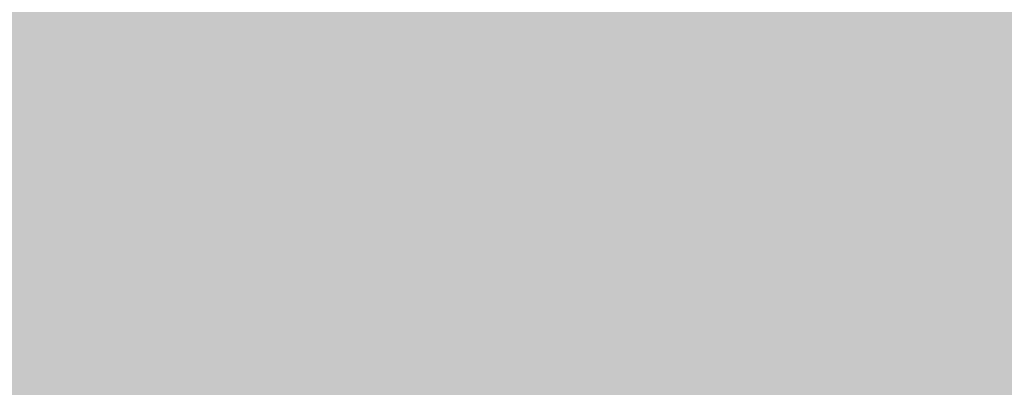
# Model space of a CAD drawing. Units: feet. Extents: x 3168 to 4724, y 827 to 1477.
# Tile 28 of 256: x 3261.901 to 3270.273, y 1093.654 to 1096.781. Entities that reach past the tile are written whole.
import ezdxf

# ---------------------------------------------------------------- set-up
doc = ezdxf.new("R2010")
doc.units = ezdxf.units.FT
doc.layers.add('A-ELEV-PATT', color=8, linetype='Continuous', lineweight=13)

msp = doc.modelspace()

# ---------------------------------------------------------------- hatches: boundary and pattern name
at = {"layer": 'A-ELEV-PATT'}
h = msp.add_hatch(color=256, dxfattribs=at)
h.dxf.hatch_style = 1
edge = h.paths.add_edge_path()
edge.add_ellipse((3552.9058, 979.2201), major_axis=(36.7449, 0), ratio=0.4848485, start_angle=0, end_angle=360)
edge = h.paths.add_edge_path()
edge.add_ellipse((3559.8916, 929.2523), major_axis=(36.7449, 0), ratio=0.4848485, start_angle=0, end_angle=360)
edge = h.paths.add_edge_path()
edge.add_line((3299.3168, 1198.6061), (3479.9167, 1198.6061))
edge.add_line((3479.9167, 1198.6061), (3479.9167, 1209.8686))
edge.add_spline(control_points=[(3479.9167, 1209.8686), (3464.3012, 1209.8686), (3448.6856, 1209.8686), (3410.9491, 1209.8686), (3388.8282, 1209.8686), (3355.6469, 1209.8686), (3344.5864, 1209.8686), (3327.9957, 1209.8686), (3322.4655, 1209.8686), (3314.1702, 1209.8686), (3311.4051, 1209.8686), (3307.2574, 1209.8686), (3305.8748, 1209.8686), (3303.801, 1209.8686), (3303.1097, 1209.8686), (3302.0728, 1209.8686), (3301.7272, 1209.8686), (3301.2087, 1209.8686), (3301.0359, 1209.8686), (3300.7767, 1209.8686), (3300.6903, 1209.8686), (3300.5606, 1209.8686), (3300.5174, 1209.8686), (3300.4526, 1209.8686), (3300.431, 1209.8686), (3300.3986, 1209.8686), (3300.3878, 1209.8686), (3300.3662, 1209.8686), (3300.3457, 1209.8686), (3300.3455, 1209.8686), (3300.3455, 1209.8686), (3300.3433, 1209.8686), (3300.3411, 1209.8686), (3300.3379, 1209.8686), (3300.3368, 1209.8686), (3300.3339, 1209.8686), (3300.3321, 1209.8686), (3300.3255, 1209.8686), (3300.3207, 1209.8686), (3300.3109, 1209.8686), (3300.306, 1209.8686), (3300.2905, 1209.8686), (3300.28, 1209.8686), (3300.2324, 1209.8688), (3300.1953, 1209.869), (3299.9511, 1209.8706), (3299.7448, 1209.8743), (3299.4368, 1209.8833), (3299.3344, 1209.8868), (3299.1811, 1209.8929), (3299.13, 1209.8951), (3298.6522, 1209.9168), (3298.2295, 1209.9457), (3297.6016, 1210.0024), (3297.3934, 1210.0235), (3297.0827, 1210.0583), (3296.9793, 1210.0705), (3296.293, 1210.1549), (3295.7181, 1210.2434), (3294.8687, 1210.3989), (3294.5877, 1210.4545), (3294.1693, 1210.5433), (3294.0304, 1210.5739), (3291.7071, 1211.1012), (3289.6536, 1211.8134), (3285.7763, 1213.564), (3283.9514, 1214.6035), (3280.5122, 1216.9801), (3278.8972, 1218.3176), (3276.3799, 1220.8295), (3275.416, 1221.9177), (3274.0393, 1223.7077), (3273.581, 1224.3495), (3273.1432, 1225.0163)], knot_values=[39.119033, 39.119033, 39.119033, 39.119033, 39.286353, 39.286353, 39.523379, 39.523379, 39.641892, 39.641892, 39.701148, 39.701148, 39.730777, 39.730777, 39.745591, 39.745591, 39.752998, 39.752998, 39.756701, 39.756701, 39.758553, 39.758553, 39.759479, 39.759479, 39.759942, 39.759942, 39.760173, 39.760173, 39.760289, 39.760289, 39.760405, 39.760405, 39.760463, 39.760463, 39.763389, 39.763389, 39.764851, 39.764851, 39.767304, 39.767304, 39.773825, 39.773825, 39.78057, 39.78057, 39.79477, 39.79477, 39.845194, 39.845194, 40.126715, 40.126715, 40.267476, 40.267476, 40.337856, 40.337856, 40.927023, 40.927023, 41.221606, 41.221606, 41.368898, 41.368898, 42.202622, 42.202622, 42.619485, 42.619485, 42.827916, 42.827916, 46.118323, 46.118323, 49.408731, 49.408731, 52.699139, 52.699139, 54.927489, 54.927489, 56.104228, 56.104228, 56.104228, 56.104228], weights=[1, 1, 1, 1, 1, 1, 1, 1, 1, 1, 1, 1, 1, 1, 1, 1, 1, 1, 1, 1, 1, 1, 1, 1, 1, 1, 1, 1, 1, 1, 1, 1, 1, 1, 1, 1, 1, 1, 1, 1, 1, 1, 1, 1, 1, 1, 1, 1, 1, 1, 1, 1, 1, 1, 1, 1, 1, 1, 1, 1, 1, 1, 1, 1, 1, 1, 1, 1, 1, 1, 1, 1, 1, 1], degree=3, periodic=0)
edge.add_line((3273.1432, 1225.0163), (3273.1432, 1099.0163))
edge.add_line((3273.1432, 1099.0163), (3299.3168, 1099.0163))
edge.add_line((3299.3168, 1099.0163), (3299.3168, 1198.6061))
edge = h.paths.add_edge_path()
edge.add_line((3304.7584, 1324.1581), (3479.9167, 1324.1581))
edge.add_line((3479.9167, 1324.1581), (3479.9167, 1335.7146))
edge.add_line((3479.9167, 1335.7146), (3269.1616, 1335.7146))
edge.add_spline(control_points=[(3269.1616, 1335.7146), (3264.0242, 1335.7146), (3258.3641, 1328.9582), (3259.2643, 1323.9003)], knot_values=[0, 0, 0, 0, 15.412191, 15.412191, 15.412191, 15.412191], degree=3, periodic=0)
edge.add_line((3259.2643, 1323.9003), (3265.5168, 1288.7691))
edge.add_line((3265.5168, 1288.7691), (3275.2651, 1261.5456))
edge.add_line((3275.2651, 1261.5456), (3304.7584, 1261.5456))
edge.add_line((3304.7584, 1261.5456), (3304.7584, 1324.1581))
h = msp.add_hatch(color=256, dxfattribs=at)
h.dxf.hatch_style = 1
h.paths.add_polyline_path([(3384.5252, 1099.0163), (3335.0292, 1099.0163), (3299.3168, 1099.0163), (3273.1432, 1099.0163), (3217.5654, 1099.0163), (3168.0693, 827.1163), (3335.0292, 827.1163)])

doc.saveas('drawing.dxf')
